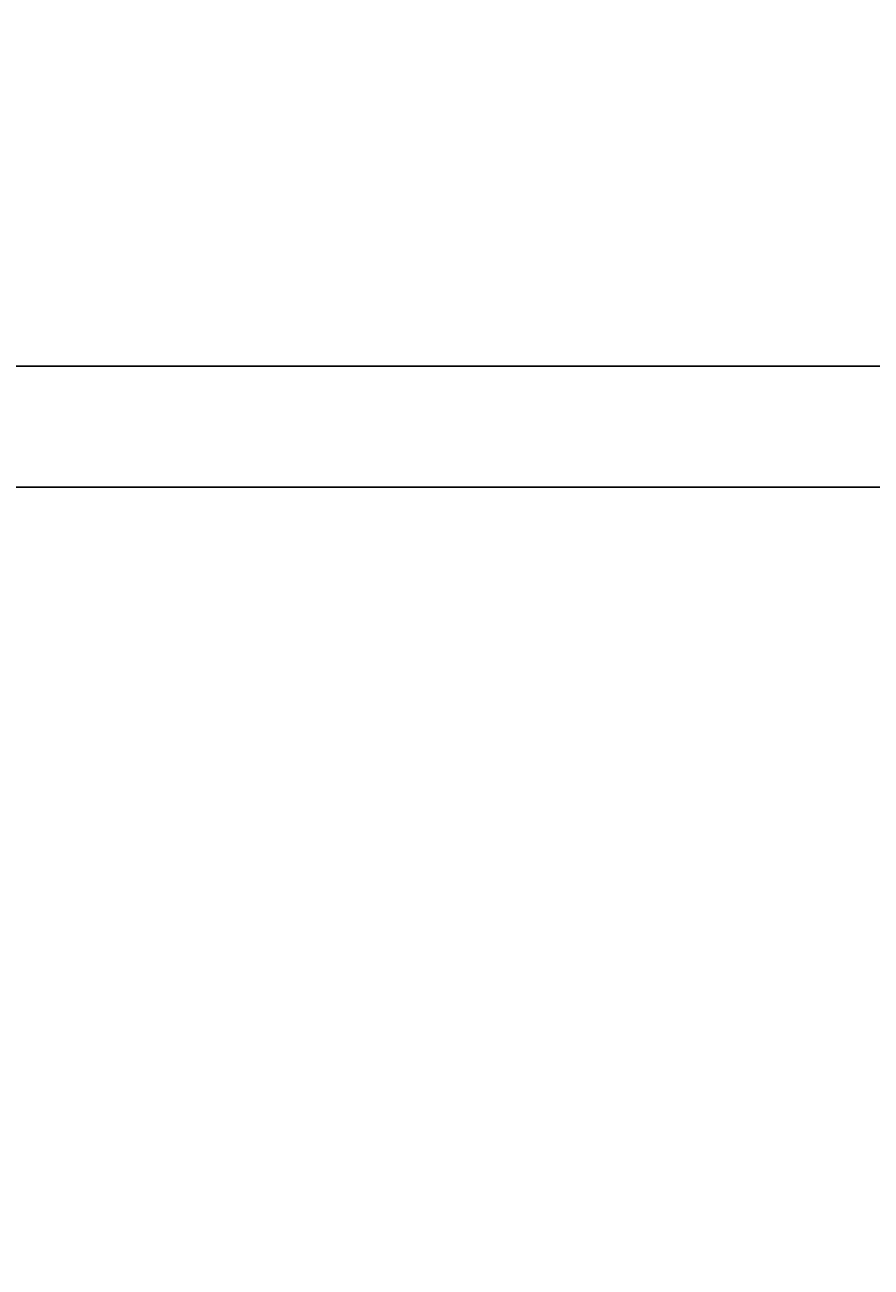
# Model space of a CAD drawing. Units: inches. Extents: x -12 to 334, y -10 to 186.
# Tile 24 of 77: x 88 to 106, y 109 to 135. Entities that reach past the tile are written whole.
import ezdxf
from ezdxf import colors
from ezdxf.entities.mleader import LeaderData, LeaderLine
from ezdxf.math import Vec2, Vec3

# ---------------------------------------------------------------- set-up
doc = ezdxf.new("R2010")
doc.units = ezdxf.units.IN
doc.header["$MEASUREMENT"] = 0
doc.layers.add('M-ANNO-TEXT', color=3, linetype='Continuous', lineweight=25)
doc.layers.add('M-DIMS', color=2, linetype='Continuous', lineweight=18)
doc.styles.get("Standard").update_dxf_attribs({"font": 'arial.ttf'})
doc.dimstyles.get("Standard").update_dxf_attribs({"dimtxt": 0.18, "dimasz": 0.18, "dimexe": 0.18, "dimexo": 0.0625, "dimgap": 0.09, "dimtad": 0, "dimtih": 1, "dimtoh": 1, "dimdec": 4, "dimzin": 0, "dimdsep": 46, "dimtxsty": 'Standard', "dimcen": 0.09, "dimadec": 0, "dimazin": 0, "dimtfac": 1, "dimtdec": 4, "dimtofl": 0, "dimtmove": 0, "dimatfit": 3, "dimfxl": 1, "dimtolj": 1, "dimtzin": 0, "dimarcsym": 0})

# ---------------------------------------------------------------- blocks, each defined once
blk = doc.blocks.new('*D5')
at = {"layer": 'Defpoints', "color": 0, "transparency": 16777216}
for p in [(58.1, 127.708), (58.1, 125.208), (295.976, 125.208)]:
    blk.add_point(p, dxfattribs=at)
at = {"layer": 'M-DIMS', "color": 0, "lineweight": -2, "transparency": 16777216}
for p, q in [((58.163, 127.708), (296.156, 127.708)), ((295.976, 127.528), (295.976, 126.64)), ((295.976, 125.388), (295.976, 126.276)), ((58.163, 125.208), (296.156, 125.208))]:
    blk.add_line(p, q, dxfattribs=at)
at = {"layer": 'M-DIMS', "color": 0, "transparency": 16777216}
for points in [[(295.946, 127.528), (296.006, 127.528), (295.976, 127.708)], [(295.946, 125.388), (296.006, 125.388), (295.976, 125.208)]]:
    blk.add_solid(points, dxfattribs=at)
at = {"layer": 'M-DIMS', "color": 0, "transparency": 16777216, "insert": (295.976, 126.458), "char_height": 0.18, "attachment_point": 5}
blk.add_mtext('\\A1;2.5', dxfattribs=at)
blk = doc.blocks.new('*D15')
at = {"layer": 'Defpoints', "color": 0, "transparency": 16777216}
for p in [(106.177, 169.385), (86.888, 109.058), (106.177, 102.896)]:
    blk.add_point(p, dxfattribs=at)
at = {"layer": 'M-DIMS', "color": 0, "lineweight": -2, "transparency": 16777216}
for p, q in [((86.888, 109.121), (86.888, 169.565)), ((106.177, 102.958), (106.177, 169.565)), ((87.068, 169.385), (96.147, 169.385)), ((105.997, 169.385), (96.918, 169.385))]:
    blk.add_line(p, q, dxfattribs=at)
at = {"layer": 'M-DIMS', "color": 0, "transparency": 16777216}
for points in [[(87.068, 169.415), (87.068, 169.355), (86.888, 169.385)], [(105.997, 169.415), (105.997, 169.355), (106.177, 169.385)]]:
    blk.add_solid(points, dxfattribs=at)
at = {"layer": 'M-DIMS', "color": 0, "transparency": 16777216, "insert": (96.532, 169.385), "char_height": 0.18, "attachment_point": 5}
blk.add_mtext('\\A1;19.29', dxfattribs=at)

msp = doc.modelspace()

# ---------------------------------------------------------------- dimensions: what is measured, and where the dimension line sits
at = {"layer": 'M-DIMS'}
dim = msp.add_linear_dim(base=(106.1771, 169.3845), p1=(86.8879, 109.0583), p2=(106.1771, 102.8958), dimstyle='Standard', override={"dimdec": 2, "dimlfac": 1, "dimrnd": 0, "dimzin": 0, "dimdsep": 46, "dimlunit": 2}, dxfattribs=at)
dim.commit()
dim.dimension.update_dxf_attribs({"geometry": '*D15', "text_midpoint": (96.5325, 169.3845)})
dim = msp.add_linear_dim(base=(295.9756, 125.2078), p1=(58.1002, 127.7078), p2=(58.1002, 125.2078), angle=90, dimstyle='Standard', override={"dimdec": 1, "dimlfac": 1, "dimrnd": 0, "dimzin": 0, "dimdsep": 46, "dimlunit": 2}, dxfattribs=at)
dim.commit()
dim.dimension.update_dxf_attribs({"geometry": '*D5', "text_midpoint": (295.9756, 126.4578)})

# ---------------------------------------------------------------- leaders
at = {"layer": 'M-ANNO-TEXT'}
ml = msp.add_multileader_mtext('Standard', dxfattribs=at)
ml.set_content('Tube plate', color=256)
ml.set_leader_properties()
ml.build(insert=Vec2(0, 0))
ml.multileader.update_dxf_attribs({"dogleg_length": 0.36, "arrow_head_size": 0.7})
ctx = ml.context
ctx.base_point, ctx.arrow_head_size, ctx.landing_gap_size, ctx.plane_origin = Vec3(95.9742, 157.4218), 0.7, 0.09, Vec3(31.4743, 171.7024)
notes = []
notes.append((ctx, [(0, (1, 1, 0), (78.5354, 157.4218), (1, 0), 17.4388, [(0, [(75.9244, 109.0583)], 0, [])])]))
ctx.mtext.insert, ctx.mtext.flow_direction = Vec3(96.0642, 159.9771), 5
for ctx, leaders in notes:
    for number, flags, end, landing, length, lines in leaders:
        leader = LeaderData()
        leader.index, (leader.has_last_leader_line, leader.has_dogleg_vector, leader.attachment_direction) = number, flags
        leader.last_leader_point, leader.dogleg_vector, leader.dogleg_length = Vec3(end), Vec3(landing), length
        for number, points, colour, breaks in lines:
            line = LeaderLine()
            line.index, line.vertices, line.color, line.breaks = number, Vec3.list(points), colors.encode_raw_color(colour), breaks
            leader.lines.append(line)
        ctx.leaders.append(leader)

doc.saveas('drawing.dxf')
